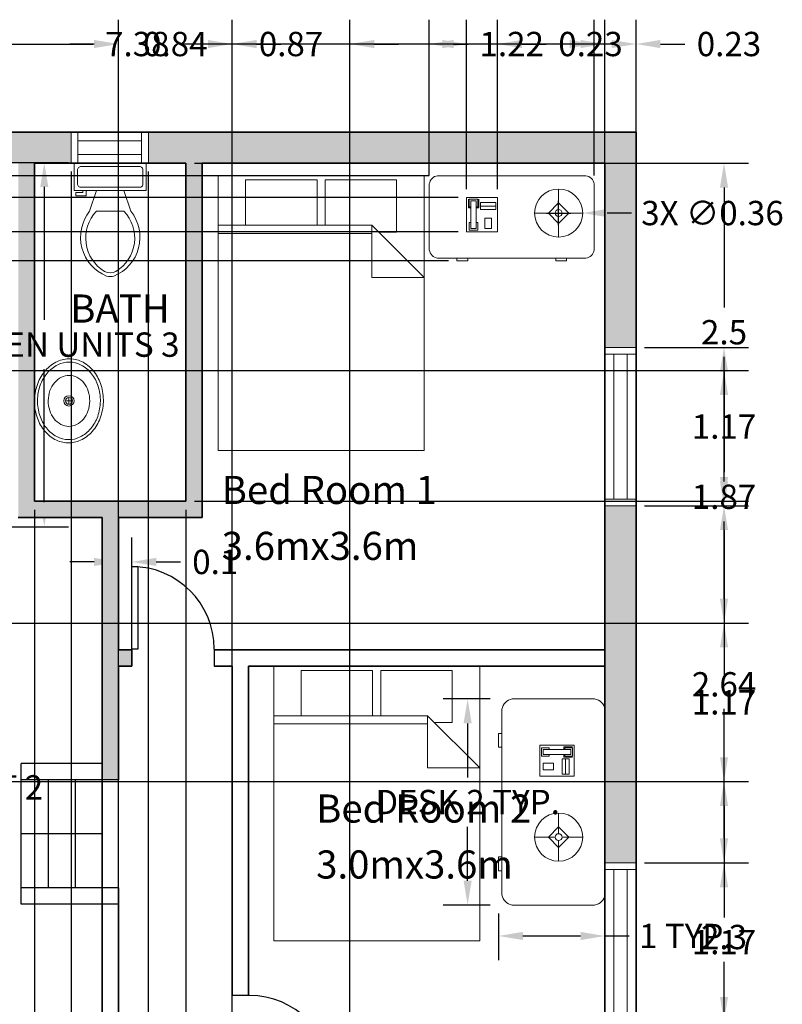
# Model space of a CAD drawing. Units: metres. Extents: x 35.2 to 46.4, y 446.1 to 460.8.
# Tile 6 of 6: x 40.4 to 46.1, y 453.5 to 460.8. Entities that reach past the tile are written whole.
import ezdxf

# ---------------------------------------------------------------- set-up
doc = ezdxf.new("R2010")
doc.units = ezdxf.units.M
for name, color, linetype, lineweight in [('A-ANNO-DIMS', 2, 'Continuous', 18), ('A-AREA-IDEN', 7, 'Continuous', 18), ('A-DOOR', 3, 'Continuous', 25), ('A-EQPM', 8, 'Continuous', 13), ('A-FLOR-STRS', 7, 'Continuous', 25), ('A-GLAZ', 4, 'Continuous', 18), ('A-WALL', 7, 'Continuous', 35), ('A-WALL-PATT', 252, 'Continuous', 13), ('FURNITURE', 53, 'Continuous', 18), ('SANITARY', 151, 'Continuous', 18)]:
    doc.layers.add(name, color=color, linetype=linetype, lineweight=lineweight)
doc.styles.get("Standard").update_dxf_attribs({"font": 'calibri.ttf'})
doc.dimstyles.get("Standard").update_dxf_attribs({"dimtxt": 0.18, "dimasz": 0.18, "dimexe": 0.18, "dimexo": 0.0625, "dimgap": 0.09, "dimtad": 0, "dimtih": 1, "dimtoh": 1, "dimdec": 4, "dimzin": 0, "dimdsep": 46, "dimtxsty": 'Standard', "dimcen": 0.09, "dimadec": 0, "dimazin": 0, "dimtfac": 1, "dimtdec": 4, "dimtofl": 0, "dimtmove": 0, "dimatfit": 3, "dimfxl": 1, "dimtolj": 1, "dimtzin": 0, "dimarcsym": 0})

# ---------------------------------------------------------------- blocks, each defined once
blk = doc.blocks.new('*U2')
for p, q in [((0, 0), (0, -5)), ((24, 0), (24, -5))]:
    blk.add_line(p, q)
blk.add_lwpolyline([(0, 0), (0, 24), (1.75, 24), (1.75, 0)], close=True)
blk.add_arc((0, 0), 24, 0, 90)
blk = doc.blocks.new('Bed - Queen')
for p, q in [((0, -80.00003), (0, 0)), ((0, 0), (59.99999, 0)), ((59.99999, 0), (59.99999, -80.00003)), ((7.99999, -1.2), (28.79998, -1.2)), ((7.99999, -14.4), (7.99999, -1.2)), ((28.79998, -1.2), (28.79998, -14.4)), ((31.19999, -1.2), (51.99999, -1.2)), ((31.19999, -14.4), (31.19999, -1.2)), ((51.99999, -1.2), (51.99999, -16.4)), ((0, -14.4), (44.8, -14.4)), ((44.8, -16.8), (0, -16.8)), ((59.99999, -29.6), (44.8, -14.4)), ((44.8, -14.4), (44.8, -29.6)), ((51.99999, -16.4), (46.79936, -16.4)), ((44.8, -29.6), (59.99999, -29.6)), ((59.99999, -80.00003), (0, -80.00003))]:
    blk.add_line(p, q)
blk = doc.blocks.new('Desk - 30 x 60 in.')
for p, q in [((-26.999995, 0), (26.999995, 0)), ((-29.999995, -27), (-29.999995, -3)), ((29.999995, -3), (29.999995, -27)), ((26.999995, -30), (-26.999995, -30)), ((-20.000005, -30), (-20.000005, -31)), ((-20.000005, -31), (-16.000005, -31)), ((-16.000005, -31), (-16.000005, -30)), ((15.999995, -31), (15.999995, -30)), ((19.999995, -31), (15.999995, -31)), ((19.999995, -30), (19.999995, -31))]:
    blk.add_line(p, q)
for centre, start, end in [((-26.499995, -3.5), 98.1301, 171.8699), ((26.499995, -3.5), 8.130102, 81.8699), ((-26.499995, -26.5), 188.1301, 261.8699), ((26.499995, -26.5), 278.1301, 351.8699)]:
    blk.add_arc(centre, 3.535534, start, end)
blk = doc.blocks.new('Lamp - Table')
for p, q in [((0, 7), (0, 1)), ((0, 3), (-3, 0)), ((3, 0), (0, 3)), ((-1, 0), (-7, 0)), ((-3, 0), (0, -3)), ((0, -3), (3, 0)), ((1, 0), (7, 0)), ((0, -1), (0, -7))]:
    blk.add_line(p, q)
for radius in [7, 1]:
    blk.add_circle((0, 0), radius)
blk = doc.blocks.new('Phone - Desk')
for p, q in [((-4.5, -5), (-4.5, 5)), ((-4.5, 5), (4.5, 5)), ((-4, 4.5), (-4, 2)), ((-3.75, 4.5), (-3.75, 2.25)), ((-1.25, 4.5), (-3.75, 4.5)), ((-3.25, 4), (-3.25, -4)), ((-3.25, 4), (-1.75, 4)), ((-1.75, -4), (-1.75, 4)), ((-1.25, 2.25), (-1.25, 4.5)), ((-1, 2), (-1, 4.5)), ((4, 3.5), (-0.5, 3.5)), ((-0.5, 3.5), (-0.5, 1.5)), ((4, 1.5), (4, 3.5)), ((4.5, 5), (4.5, -5)), ((-4, 2), (-3.25, 2)), ((-3.75, 2.25), (-3.25, 2.25)), ((-1.75, 2.25), (-1.25, 2.25)), ((-1.75, 2), (-1, 2)), ((-0.5, 2.5), (4, 2.5)), ((-0.5, 1.5), (4, 1.5)), ((-3.75, -2.25), (-3.25, -2.25)), ((-3.75, -4.5), (-3.75, -2.25)), ((-1.75, -2.25), (-1.25, -2.25)), ((-1.25, -2.25), (-1.25, -4.5)), ((2.75, -1), (0.75, -1)), ((0.75, -1), (0.75, -4)), ((2.75, -4), (2.75, -1)), ((4.5, -5), (-4.5, -5)), ((-1.25, -4.5), (-3.75, -4.5)), ((-3.25, -4), (-1.75, -4)), ((0.75, -4), (2.75, -4))]:
    blk.add_line(p, q)
blk = doc.blocks.new('Toilet - top')
for p, q in [((9.5, -6), (9.5, -2)), ((-10, -8.5), (-8, -8.5)), ((-10, -9.5), (-10, -8.5)), ((-8, -8.5), (-8, -8)), ((-7, -8), (-7, -9.5)), ((-4, -8), (-6, -14)), ((4, -8), (6, -14)), ((-7, -9.5), (-10, -9.5)), ((4, -14), (-4, -14))]:
    blk.add_line(p, q)
blk.add_lwpolyline([(10.5, -8), (10.5, 0), (-10.5, 0), (-10.5, -8)], close=True)
for points in [[(-9.5, -2), (-9.5, -6)], [(8.5, -1), (-8.5, -1)], [(-8.5, -7), (8.5, -7)]]:
    blk.add_lwpolyline(points)
for centre, radius, start, end in [((-8.62, -1.88), 0.884, 81.8699, 188.1301), ((8.62, -1.88), 0.884, 351.8699, 98.1301), ((-8.62, -6.12), 0.884, 171.8699, 278.1301), ((8.62, -6.12), 0.884, 261.8699, 8.1301), ((3.52, -21.58), 12.17, 141.4691, 247.9714), ((4.2, -21.82), 11.33, 136.3677, 238.9468), ((-3.52, -21.58), 12.17, 292.0284, 38.5307), ((-4.2, -21.82), 11.33, 301.053, 43.6321), ((0, -27.88), 4, 245.7318, 294.2682), ((0, -29), 4, 254.8605, 285.1395)]:
    blk.add_arc(centre, radius, start, end)
blk = doc.blocks.new('Sink - Oval top')
for p, q in [((-1, 0), (1, 0)), ((0, 1), (0, -1))]:
    blk.add_line(p, q)
for points in [[(-12.23, 0.39, 0.117634), (-11.46, -3.36, 0.104469), (-8.88, -6.8, 0.090016), (-5.08, -9.07, 0.08192), (-0.32, -10.02, 0.08192), (4.49, -9.38, 0.090016), (8.42, -7.36, 0.104469), (11.22, -4.09, 0.117634), (12.23, -0.39, 0.117634), (11.46, 3.36, 0.104469), (8.88, 6.8, 0.090016), (5.08, 9.07, 0.08192), (0.32, 10.02, 0.08192), (-4.49, 9.38, 0.090016), (-8.42, 7.36, 0.104469), (-11.22, 4.09, 0.117634)], [(-11.29, 0.16, 0.118622), (-10.52, -3.25, 0.104678), (-8.07, -6.36, 0.089562), (-4.54, -8.37, 0.081185), (-0.13, -9.15, 0.081185), (4.3, -8.49, 0.089562), (7.89, -6.58, 0.104678), (10.42, -3.55, 0.118622), (11.29, -0.16, 0.118622), (10.52, 3.25, 0.104678), (8.07, 6.36, 0.089562), (4.54, 8.37, 0.081185), (0.13, 9.15, 0.081185), (-4.3, 8.49, 0.089562), (-7.89, 6.58, 0.104678), (-10.42, 3.55, 0.118622)], [(-7.42, 0.08, 0.118283), (-6.91, -2.17, 0.104607), (-5.29, -4.21, 0.089718), (-2.97, -5.53, 0.081436), (-0.07, -6.04, 0.081436), (2.84, -5.59, 0.089718), (5.2, -4.33, 0.104607), (6.86, -2.32, 0.118283), (7.42, -0.08, 0.118283), (6.91, 2.17, 0.104607), (5.29, 4.21, 0.089718), (2.97, 5.53, 0.081436), (0.07, 6.04, 0.081436), (-2.84, 5.59, 0.089718), (-5.2, 4.33, 0.104607), (-6.86, 2.32, 0.118283)]]:
    blk.add_lwpolyline(points, format="xyb", close=True)
for radius in [1.5, 1]:
    blk.add_circle((0, 0), radius)
blk = doc.blocks.new('*U3')
for p, q in [((0, 0), (0, 5)), ((24, 0), (24, 5))]:
    blk.add_line(p, q)
blk.add_lwpolyline([(0, 0), (0, -24), (1.75, -24), (1.75, 0)], close=True)
blk.add_arc((0, 0), 24, 270, 0)
blk = doc.blocks.new('WIN-1172')
for p, q in [((0, 1.1716), (0.23, 1.1716)), ((0, 1.1716), (0, 0)), ((0.23, 1.1716), (0.23, 0)), ((0, 1.1216), (0.23, 1.1216)), ((0.065, 1.1216), (0.065, 0.05)), ((0.165, 1.1216), (0.165, 0.05)), ((0.23, 0.05), (0, 0.05)), ((0.23, 0), (0, 0))]:
    blk.add_line(p, q)
blk = doc.blocks.new('WIN-572')
for p, q in [((0, 0.5716), (0.23, 0.5716)), ((0, 0.5716), (0, 0)), ((0, 0.5216), (0.23, 0.5216)), ((0.065, 0.5216), (0.065, 0.05)), ((0.165, 0.5216), (0.165, 0.05)), ((0.23, 0.5716), (0.23, 0)), ((0.23, 0.05), (0, 0.05)), ((0.23, 0), (0, 0))]:
    blk.add_line(p, q)
blk = doc.blocks.new('*D133')
at = {"layer": 'A-ANNO-DIMS', "color": 0, "lineweight": -2, "transparency": 16777216}
for p, q in [((43.9067, 455.7324), (43.5606, 455.7324)), ((43.7406, 455.5524), (43.7406, 455.1526)), ((43.7406, 454.3884), (43.7406, 454.7882)), ((43.9067, 454.2084), (43.5606, 454.2084))]:
    blk.add_line(p, q, dxfattribs=at)
at = {"layer": 'A-ANNO-DIMS', "color": 0, "transparency": 16777216}
for points in [[(43.7106, 455.5524), (43.7706, 455.5524), (43.7406, 455.7324)], [(43.7106, 454.3884), (43.7706, 454.3884), (43.7406, 454.2084)]]:
    blk.add_solid(points, dxfattribs=at)
at = {"layer": 'Defpoints', "color": 0, "transparency": 16777216}
for p in [(43.9692, 455.7324), (43.7406, 454.2084), (43.9692, 454.2084)]:
    blk.add_point(p, dxfattribs=at)
at = {"layer": 'A-ANNO-DIMS', "color": 0, "transparency": 16777216, "insert": (43.7406, 454.9704), "char_height": 0.18, "attachment_point": 5}
blk.add_mtext('\\A1;DESK 2 TYP.', dxfattribs=at)
blk = doc.blocks.new('*D134')
at = {"layer": 'A-ANNO-DIMS', "color": 0, "lineweight": -2, "transparency": 16777216}
for p, q in [((43.9692, 454.1459), (43.9692, 453.7998)), ((44.7566, 454.1459), (44.7566, 453.7998)), ((44.1492, 453.9798), (44.5766, 453.9798)), ((44.7566, 453.9798), (44.9366, 453.9798))]:
    blk.add_line(p, q, dxfattribs=at)
at = {"layer": 'A-ANNO-DIMS', "color": 0, "transparency": 16777216}
for points in [[(44.1492, 454.0098), (44.1492, 453.9498), (43.9692, 453.9798)], [(44.5766, 454.0098), (44.5766, 453.9498), (44.7566, 453.9798)]]:
    blk.add_solid(points, dxfattribs=at)
at = {"layer": 'Defpoints', "color": 0, "transparency": 16777216}
for p in [(43.9692, 454.2084), (44.7566, 454.2084), (44.7566, 453.9798)]:
    blk.add_point(p, dxfattribs=at)
at = {"layer": 'A-ANNO-DIMS', "color": 0, "transparency": 16777216, "insert": (45.3552, 453.9798), "char_height": 0.18, "attachment_point": 5}
blk.add_mtext('\\A1;1 TYP.', dxfattribs=at)
blk = doc.blocks.new('*D139')
at = {"layer": 'A-ANNO-DIMS', "color": 0, "lineweight": -2, "transparency": 16777216}
for p, q in [((39.5553, 456.2345), (40.0195, 456.2345)), ((39.8395, 456.0545), (39.8395, 455.261)), ((39.8395, 454.1031), (39.8395, 454.8966)), ((39.5553, 453.9231), (40.0195, 453.9231))]:
    blk.add_line(p, q, dxfattribs=at)
at = {"layer": 'A-ANNO-DIMS', "color": 0, "transparency": 16777216}
for points in [[(39.8095, 456.0545), (39.8695, 456.0545), (39.8395, 456.2345)], [(39.8095, 454.1031), (39.8695, 454.1031), (39.8395, 453.9231)]]:
    blk.add_solid(points, dxfattribs=at)
at = {"layer": 'Defpoints', "color": 0, "transparency": 16777216}
for p in [(39.4928, 456.2345), (39.8395, 456.2345), (39.4928, 453.9231)]:
    blk.add_point(p, dxfattribs=at)
at = {"layer": 'A-ANNO-DIMS', "color": 0, "transparency": 16777216, "insert": (39.8395, 455.0788), "char_height": 0.18, "attachment_point": 5}
blk.add_mtext('\\A1;DINING SET 2', dxfattribs=at)
blk = doc.blocks.new('*D145')
at = {"layer": 'A-ANNO-DIMS', "color": 0, "lineweight": -2, "transparency": 16777216}
for p, q in [((40.2671, 459.6992), (40.7885, 459.6992)), ((40.6085, 459.5192), (40.6085, 458.5353)), ((40.6085, 457.1868), (40.6085, 458.1708)), ((40.2671, 457.0068), (40.7885, 457.0068))]:
    blk.add_line(p, q, dxfattribs=at)
at = {"layer": 'A-ANNO-DIMS', "color": 0, "transparency": 16777216}
for points in [[(40.5785, 459.5192), (40.6385, 459.5192), (40.6085, 459.6992)], [(40.5785, 457.1868), (40.6385, 457.1868), (40.6085, 457.0068)]]:
    blk.add_solid(points, dxfattribs=at)
at = {"layer": 'Defpoints', "color": 0, "transparency": 16777216}
for p in [(40.2046, 459.6992), (40.6085, 459.6992), (40.2046, 457.0068)]:
    blk.add_point(p, dxfattribs=at)
at = {"layer": 'A-ANNO-DIMS', "color": 0, "transparency": 16777216, "insert": (40.6085, 458.353), "char_height": 0.18, "attachment_point": 5}
blk.add_mtext('\\A1;KITCHEN UNITS 3', dxfattribs=at)
blk = doc.blocks.new('*D151')
at = {"layer": 'A-ANNO-DIMS', "color": 0, "lineweight": -2, "transparency": 16777216}
for p, q in [((37.6066, 459.9873), (37.6066, 460.756)), ((44.9866, 459.9873), (44.9866, 460.756)), ((37.7866, 460.576), (40.9679, 460.576)), ((44.8066, 460.576), (41.6253, 460.576))]:
    blk.add_line(p, q, dxfattribs=at)
at = {"layer": 'A-ANNO-DIMS', "color": 0, "transparency": 16777216}
for points in [[(37.7866, 460.606), (37.7866, 460.546), (37.6066, 460.576)], [(44.8066, 460.606), (44.8066, 460.546), (44.9866, 460.576)]]:
    blk.add_solid(points, dxfattribs=at)
at = {"layer": 'Defpoints', "color": 0, "transparency": 16777216}
for p in [(44.9866, 460.576), (37.6066, 459.9248), (44.9866, 459.9248)]:
    blk.add_point(p, dxfattribs=at)
at = {"layer": 'A-ANNO-DIMS', "color": 0, "transparency": 16777216, "insert": (41.2966, 460.576), "char_height": 0.18, "attachment_point": 5}
blk.add_mtext('\\A1;7.38', dxfattribs=at)
blk = doc.blocks.new('*D156')
at = {"layer": 'A-ANNO-DIMS', "color": 0, "lineweight": -2, "transparency": 16777216}
for p, q in [((37.8991, 455.122), (45.8178, 455.122)), ((45.6378, 454.942), (45.6378, 454.1543)), ((45.6378, 453.0022), (45.6378, 453.7898)), ((37.8991, 452.8222), (45.8178, 452.8222))]:
    blk.add_line(p, q, dxfattribs=at)
at = {"layer": 'A-ANNO-DIMS', "color": 0, "transparency": 16777216}
for points in [[(45.6078, 454.942), (45.6678, 454.942), (45.6378, 455.122)], [(45.6078, 453.0022), (45.6678, 453.0022), (45.6378, 452.8222)]]:
    blk.add_solid(points, dxfattribs=at)
at = {"layer": 'Defpoints', "color": 0, "transparency": 16777216}
for p in [(37.8366, 455.122), (45.6378, 455.122), (37.8366, 452.8222)]:
    blk.add_point(p, dxfattribs=at)
at = {"layer": 'A-ANNO-DIMS', "color": 0, "transparency": 16777216, "insert": (45.6378, 453.9721), "char_height": 0.18, "attachment_point": 5}
blk.add_mtext('\\A1;2.3', dxfattribs=at)
blk = doc.blocks.new('*D157')
at = {"layer": 'A-ANNO-DIMS', "color": 0, "lineweight": -2, "transparency": 16777216}
for p, q in [((37.8991, 456.2935), (45.8178, 456.2935)), ((45.6378, 456.1135), (45.6378, 455.8886)), ((45.6378, 455.302), (45.6378, 455.5269)), ((37.8991, 455.122), (45.8178, 455.122))]:
    blk.add_line(p, q, dxfattribs=at)
at = {"layer": 'A-ANNO-DIMS', "color": 0, "transparency": 16777216}
for points in [[(45.6078, 456.1135), (45.6678, 456.1135), (45.6378, 456.2935)], [(45.6078, 455.302), (45.6678, 455.302), (45.6378, 455.122)]]:
    blk.add_solid(points, dxfattribs=at)
at = {"layer": 'Defpoints', "color": 0, "transparency": 16777216}
for p in [(37.8366, 456.2935), (45.6378, 456.2935), (37.8366, 455.122)]:
    blk.add_point(p, dxfattribs=at)
at = {"layer": 'A-ANNO-DIMS', "color": 0, "transparency": 16777216, "insert": (45.6378, 455.7077), "char_height": 0.18, "attachment_point": 5}
blk.add_mtext('\\A1;1.17', dxfattribs=at)
blk = doc.blocks.new('*D158')
at = {"layer": 'A-ANNO-DIMS', "color": 0, "lineweight": -2, "transparency": 16777216}
for p, q in [((37.8991, 458.1617), (45.8178, 458.1617)), ((45.6378, 457.9817), (45.6378, 457.4098)), ((45.6378, 456.4735), (45.6378, 457.0454)), ((37.8991, 456.2935), (45.8178, 456.2935))]:
    blk.add_line(p, q, dxfattribs=at)
at = {"layer": 'A-ANNO-DIMS', "color": 0, "transparency": 16777216}
for points in [[(45.6078, 457.9817), (45.6678, 457.9817), (45.6378, 458.1617)], [(45.6078, 456.4735), (45.6678, 456.4735), (45.6378, 456.2935)]]:
    blk.add_solid(points, dxfattribs=at)
at = {"layer": 'Defpoints', "color": 0, "transparency": 16777216}
for p in [(37.8366, 458.1617), (45.6378, 458.1617), (37.8366, 456.2935)]:
    blk.add_point(p, dxfattribs=at)
at = {"layer": 'A-ANNO-DIMS', "color": 0, "transparency": 16777216, "insert": (45.6378, 457.2276), "char_height": 0.18, "attachment_point": 5}
blk.add_mtext('\\A1;1.87', dxfattribs=at)
blk = doc.blocks.new('*D164')
at = {"layer": 'A-ANNO-DIMS', "color": 0, "lineweight": -2, "transparency": 16777216}
for p, q in [((45.0491, 454.5208), (45.8178, 454.5208)), ((45.6378, 454.3408), (45.6378, 454.1159)), ((45.6378, 453.5293), (45.6378, 453.7542)), ((45.0491, 453.3493), (45.8178, 453.3493))]:
    blk.add_line(p, q, dxfattribs=at)
at = {"layer": 'A-ANNO-DIMS', "color": 0, "transparency": 16777216}
for points in [[(45.6078, 454.3408), (45.6678, 454.3408), (45.6378, 454.5208)], [(45.6078, 453.5293), (45.6678, 453.5293), (45.6378, 453.3493)]]:
    blk.add_solid(points, dxfattribs=at)
at = {"layer": 'Defpoints', "color": 0, "transparency": 16777216}
for p in [(44.9866, 454.5208), (45.6378, 454.5208), (44.9866, 453.3493)]:
    blk.add_point(p, dxfattribs=at)
at = {"layer": 'A-ANNO-DIMS', "color": 0, "transparency": 16777216, "insert": (45.6378, 453.9351), "char_height": 0.18, "attachment_point": 5}
blk.add_mtext('\\A1;1.17', dxfattribs=at)
blk = doc.blocks.new('*D165')
at = {"layer": 'A-ANNO-DIMS', "color": 0, "lineweight": -2, "transparency": 16777216}
for p, q in [((45.0491, 457.1611), (45.8178, 457.1611)), ((45.6378, 456.9811), (45.6378, 456.0232)), ((45.6378, 454.7008), (45.6378, 455.6588)), ((45.0491, 454.5208), (45.8178, 454.5208))]:
    blk.add_line(p, q, dxfattribs=at)
at = {"layer": 'A-ANNO-DIMS', "color": 0, "transparency": 16777216}
for points in [[(45.6078, 456.9811), (45.6678, 456.9811), (45.6378, 457.1611)], [(45.6078, 454.7008), (45.6678, 454.7008), (45.6378, 454.5208)]]:
    blk.add_solid(points, dxfattribs=at)
at = {"layer": 'Defpoints', "color": 0, "transparency": 16777216}
for p in [(44.9866, 457.1611), (45.6378, 457.1611), (44.9866, 454.5208)]:
    blk.add_point(p, dxfattribs=at)
at = {"layer": 'A-ANNO-DIMS', "color": 0, "transparency": 16777216, "insert": (45.6378, 455.841), "char_height": 0.18, "attachment_point": 5}
blk.add_mtext('\\A1;2.64', dxfattribs=at)
blk = doc.blocks.new('*D166')
at = {"layer": 'A-ANNO-DIMS', "color": 0, "lineweight": -2, "transparency": 16777216}
for p, q in [((45.0491, 458.3327), (45.8178, 458.3327)), ((45.6378, 458.1527), (45.6378, 457.9277)), ((45.6378, 457.3411), (45.6378, 457.5661)), ((45.0491, 457.1611), (45.8178, 457.1611))]:
    blk.add_line(p, q, dxfattribs=at)
at = {"layer": 'A-ANNO-DIMS', "color": 0, "transparency": 16777216}
for points in [[(45.6078, 458.1527), (45.6678, 458.1527), (45.6378, 458.3327)], [(45.6078, 457.3411), (45.6678, 457.3411), (45.6378, 457.1611)]]:
    blk.add_solid(points, dxfattribs=at)
at = {"layer": 'Defpoints', "color": 0, "transparency": 16777216}
for p in [(44.9866, 458.3327), (45.6378, 458.3327), (44.9866, 457.1611)]:
    blk.add_point(p, dxfattribs=at)
at = {"layer": 'A-ANNO-DIMS', "color": 0, "transparency": 16777216, "insert": (45.6378, 457.7469), "char_height": 0.18, "attachment_point": 5}
blk.add_mtext('\\A1;1.17', dxfattribs=at)
blk = doc.blocks.new('*D167')
at = {"layer": 'A-ANNO-DIMS', "color": 0, "lineweight": -2, "transparency": 16777216}
for p, q in [((37.8366, 459.6323), (37.8366, 446.0736)), ((40.8069, 459.6323), (40.8069, 446.0736)), ((38.0166, 446.2536), (38.9948, 446.2536)), ((40.6269, 446.2536), (39.6486, 446.2536))]:
    blk.add_line(p, q, dxfattribs=at)
at = {"layer": 'A-ANNO-DIMS', "color": 0, "transparency": 16777216}
for points in [[(38.0166, 446.2836), (38.0166, 446.2236), (37.8366, 446.2536)], [(40.6269, 446.2836), (40.6269, 446.2236), (40.8069, 446.2536)]]:
    blk.add_solid(points, dxfattribs=at)
at = {"layer": 'Defpoints', "color": 0, "transparency": 16777216}
for p in [(37.8366, 459.6948), (40.8069, 459.6948), (40.8069, 446.2536)]:
    blk.add_point(p, dxfattribs=at)
at = {"layer": 'A-ANNO-DIMS', "color": 0, "transparency": 16777216, "insert": (39.3217, 446.2536), "char_height": 0.18, "attachment_point": 5}
blk.add_mtext('\\A1;2.97', dxfattribs=at)
blk = doc.blocks.new('*D168')
at = {"layer": 'A-ANNO-DIMS', "color": 0, "lineweight": -2, "transparency": 16777216}
for p, q in [((40.8069, 459.6323), (40.8069, 446.0736)), ((41.3784, 459.6323), (41.3784, 446.0736)), ((40.9869, 446.2536), (41.1984, 446.2536)), ((41.3784, 446.2536), (41.5584, 446.2536))]:
    blk.add_line(p, q, dxfattribs=at)
at = {"layer": 'A-ANNO-DIMS', "color": 0, "transparency": 16777216}
for points in [[(40.9869, 446.2836), (40.9869, 446.2236), (40.8069, 446.2536)], [(41.1984, 446.2836), (41.1984, 446.2236), (41.3784, 446.2536)]]:
    blk.add_solid(points, dxfattribs=at)
at = {"layer": 'Defpoints', "color": 0, "transparency": 16777216}
for p in [(40.8069, 459.6948), (41.3784, 459.6948), (41.3784, 446.2536)]:
    blk.add_point(p, dxfattribs=at)
at = {"layer": 'A-ANNO-DIMS', "color": 0, "transparency": 16777216, "insert": (41.8883, 446.2536), "char_height": 0.18, "attachment_point": 5}
blk.add_mtext('\\A1;0.57', dxfattribs=at)
blk = doc.blocks.new('*D169')
at = {"layer": 'A-ANNO-DIMS', "color": 0, "lineweight": -2, "transparency": 16777216}
for p, q in [((40.536595, 457.132279), (40.536595, 446.073579)), ((41.656595, 457.132279), (41.656595, 446.073579)), ((40.356595, 446.253579), (40.176595, 446.253579)), ((41.836595, 446.253579), (42.016595, 446.253579))]:
    blk.add_line(p, q, dxfattribs=at)
at = {"layer": 'A-ANNO-DIMS', "color": 0, "transparency": 16777216}
for points in [[(40.356595, 446.283579), (40.356595, 446.223579), (40.536595, 446.253579)], [(41.836595, 446.283579), (41.836595, 446.223579), (41.656595, 446.253579)]]:
    blk.add_solid(points, dxfattribs=at)
at = {"layer": 'Defpoints', "color": 0, "transparency": 16777216}
for p in [(40.536595, 457.194779), (41.656595, 457.194779), (41.656595, 446.253579)]:
    blk.add_point(p, dxfattribs=at)
at = {"layer": 'A-ANNO-DIMS', "color": 0, "transparency": 16777216, "insert": (41.096595, 446.253579), "char_height": 0.18, "attachment_point": 5}
blk.add_mtext('\\A1;1.12', dxfattribs=at)
blk = doc.blocks.new('*D170')
at = {"layer": 'A-ANNO-DIMS', "color": 0, "lineweight": -2, "transparency": 16777216}
for p, q in [((41.7191, 459.6948), (45.8178, 459.6948)), ((45.6378, 459.5148), (45.6378, 458.627)), ((45.6378, 457.3748), (45.6378, 458.2626)), ((41.7191, 457.1948), (45.8178, 457.1948))]:
    blk.add_line(p, q, dxfattribs=at)
at = {"layer": 'A-ANNO-DIMS', "color": 0, "transparency": 16777216}
for points in [[(45.6078, 459.5148), (45.6678, 459.5148), (45.6378, 459.6948)], [(45.6078, 457.3748), (45.6678, 457.3748), (45.6378, 457.1948)]]:
    blk.add_solid(points, dxfattribs=at)
at = {"layer": 'Defpoints', "color": 0, "transparency": 16777216}
for p in [(41.6566, 459.6948), (41.6566, 457.1948), (45.6378, 457.1948)]:
    blk.add_point(p, dxfattribs=at)
at = {"layer": 'A-ANNO-DIMS', "color": 0, "transparency": 16777216, "insert": (45.6378, 458.4448), "char_height": 0.18, "attachment_point": 5}
blk.add_mtext('\\A1;2.5', dxfattribs=at)
blk = doc.blocks.new('*D175')
at = {"layer": 'A-ANNO-DIMS', "color": 0, "lineweight": -2, "transparency": 16777216}
for p, q in [((44.7566, 451.1428), (44.7566, 460.756)), ((44.9866, 451.1428), (44.9866, 460.756)), ((44.5766, 460.576), (44.3966, 460.576)), ((45.1666, 460.576), (45.3466, 460.576))]:
    blk.add_line(p, q, dxfattribs=at)
at = {"layer": 'A-ANNO-DIMS', "color": 0, "transparency": 16777216}
for points in [[(44.5766, 460.606), (44.5766, 460.546), (44.7566, 460.576)], [(45.1666, 460.606), (45.1666, 460.546), (44.9866, 460.576)]]:
    blk.add_solid(points, dxfattribs=at)
at = {"layer": 'Defpoints', "color": 0, "transparency": 16777216}
for p in [(44.9866, 460.576), (44.7566, 451.0803), (44.9866, 451.0803)]:
    blk.add_point(p, dxfattribs=at)
at = {"layer": 'A-ANNO-DIMS', "color": 0, "transparency": 16777216, "insert": (45.6744, 460.576), "char_height": 0.18, "attachment_point": 5}
blk.add_mtext('\\A1;0.23', dxfattribs=at)
blk = doc.blocks.new('*D176')
at = {"layer": 'A-ANNO-DIMS', "color": 0, "lineweight": -2, "transparency": 16777216}
for p, q in [((43.7336, 459.5036), (43.7336, 460.756)), ((43.9622, 459.5036), (43.9622, 460.756)), ((43.5536, 460.576), (43.3736, 460.576)), ((44.1422, 460.576), (44.3222, 460.576))]:
    blk.add_line(p, q, dxfattribs=at)
at = {"layer": 'A-ANNO-DIMS', "color": 0, "transparency": 16777216}
for points in [[(43.5536, 460.606), (43.5536, 460.546), (43.7336, 460.576)], [(44.1422, 460.606), (44.1422, 460.546), (43.9622, 460.576)]]:
    blk.add_solid(points, dxfattribs=at)
at = {"layer": 'Defpoints', "color": 0, "transparency": 16777216}
for p in [(43.9622, 460.576), (43.7336, 459.4411), (43.9622, 459.4411)]:
    blk.add_point(p, dxfattribs=at)
at = {"layer": 'A-ANNO-DIMS', "color": 0, "transparency": 16777216, "insert": (44.65, 460.576), "char_height": 0.18, "attachment_point": 5}
blk.add_mtext('\\A1;0.23', dxfattribs=at)
blk = doc.blocks.new('*D177')
at = {"layer": 'A-ANNO-DIMS', "color": 0, "lineweight": -2, "transparency": 16777216}
for p, q in [((36.9554, 459.6211), (36.9554, 459.8011)), ((36.9554, 459.8011), (37.1354, 459.8011)), ((43.6711, 459.4411), (36.7754, 459.4411)), ((43.6711, 459.1871), (36.7754, 459.1871)), ((36.9554, 459.0071), (36.9554, 458.8271))]:
    blk.add_line(p, q, dxfattribs=at)
at = {"layer": 'A-ANNO-DIMS', "color": 0, "transparency": 16777216}
for points in [[(36.9254, 459.6211), (36.9854, 459.6211), (36.9554, 459.4411)], [(36.9254, 459.0071), (36.9854, 459.0071), (36.9554, 459.1871)]]:
    blk.add_solid(points, dxfattribs=at)
at = {"layer": 'Defpoints', "color": 0, "transparency": 16777216}
for p in [(36.9554, 459.4411), (43.7336, 459.4411), (43.7336, 459.1871)]:
    blk.add_point(p, dxfattribs=at)
at = {"layer": 'A-ANNO-DIMS', "color": 0, "transparency": 16777216, "insert": (37.5396, 459.8011), "char_height": 0.18, "attachment_point": 5}
blk.add_mtext('\\A1;0.254', dxfattribs=at)
blk = doc.blocks.new('*D178')
at = {"layer": 'A-ANNO-DIMS', "color": 0, "lineweight": -2, "transparency": 16777216}
for p, q in [((43.4574, 459.6039), (43.4574, 460.756)), ((44.6766, 459.6039), (44.6766, 460.756)), ((43.6374, 460.576), (43.7456, 460.576)), ((44.4966, 460.576), (44.3884, 460.576))]:
    blk.add_line(p, q, dxfattribs=at)
at = {"layer": 'A-ANNO-DIMS', "color": 0, "transparency": 16777216}
for points in [[(43.6374, 460.606), (43.6374, 460.546), (43.4574, 460.576)], [(44.4966, 460.606), (44.4966, 460.546), (44.6766, 460.576)]]:
    blk.add_solid(points, dxfattribs=at)
at = {"layer": 'Defpoints', "color": 0, "transparency": 16777216}
for p in [(44.6766, 460.576), (43.4574, 459.5414), (44.6766, 459.5414)]:
    blk.add_point(p, dxfattribs=at)
at = {"layer": 'A-ANNO-DIMS', "color": 0, "transparency": 16777216, "insert": (44.067, 460.576), "char_height": 0.18, "attachment_point": 5}
blk.add_mtext('\\A1;1.22', dxfattribs=at)
blk = doc.blocks.new('*D179')
at = {"layer": 'A-ANNO-DIMS', "color": 0, "lineweight": -2, "transparency": 16777216}
for p, q in [((43.4559, 459.6024), (36.7754, 459.6024)), ((36.9554, 459.4224), (36.9554, 459.1525)), ((43.5981, 458.9725), (36.7754, 458.9725)), ((36.9554, 458.9725), (36.9554, 458.7925)), ((36.9554, 458.7925), (36.7754, 458.7925))]:
    blk.add_line(p, q, dxfattribs=at)
at = {"layer": 'A-ANNO-DIMS', "color": 0, "transparency": 16777216}
for points in [[(36.9254, 459.4224), (36.9854, 459.4224), (36.9554, 459.6024)], [(36.9254, 459.1525), (36.9854, 459.1525), (36.9554, 458.9725)]]:
    blk.add_solid(points, dxfattribs=at)
at = {"layer": 'Defpoints', "color": 0, "transparency": 16777216}
for p in [(43.5184, 459.6024), (36.9554, 458.9725), (43.6606, 458.9725)]:
    blk.add_point(p, dxfattribs=at)
at = {"layer": 'A-ANNO-DIMS', "color": 0, "transparency": 16777216, "insert": (36.4476, 458.7925), "char_height": 0.18, "attachment_point": 5}
blk.add_mtext('\\A1;0.63', dxfattribs=at)
blk = doc.blocks.new('*D182')
at = {"layer": 'A-ANNO-DIMS', "color": 0, "lineweight": -2, "transparency": 16777216}
for p, q in [((41.9991, 452.3173), (41.9991, 460.756)), ((42.8695, 452.3173), (42.8695, 460.756)), ((41.8191, 460.576), (41.6391, 460.576)), ((43.0495, 460.576), (43.2295, 460.576))]:
    blk.add_line(p, q, dxfattribs=at)
at = {"layer": 'A-ANNO-DIMS', "color": 0, "transparency": 16777216}
for points in [[(41.8191, 460.606), (41.8191, 460.546), (41.9991, 460.576)], [(43.0495, 460.606), (43.0495, 460.546), (42.8695, 460.576)]]:
    blk.add_solid(points, dxfattribs=at)
at = {"layer": 'Defpoints', "color": 0, "transparency": 16777216}
for p in [(42.8695, 460.576), (41.9991, 452.2548), (42.8695, 452.2548)]:
    blk.add_point(p, dxfattribs=at)
at = {"layer": 'A-ANNO-DIMS', "color": 0, "transparency": 16777216, "insert": (42.4343, 460.576), "char_height": 0.18, "attachment_point": 5}
blk.add_mtext('\\A1;0.87', dxfattribs=at)
blk = doc.blocks.new('*D183')
at = {"layer": 'A-ANNO-DIMS', "color": 0, "lineweight": -2, "transparency": 16777216}
for p, q in [((41.1566, 450.3173), (41.1566, 460.756)), ((41.9991, 450.3173), (41.9991, 460.756)), ((40.9766, 460.576), (40.7966, 460.576)), ((42.1791, 460.576), (42.3591, 460.576))]:
    blk.add_line(p, q, dxfattribs=at)
at = {"layer": 'A-ANNO-DIMS', "color": 0, "transparency": 16777216}
for points in [[(40.9766, 460.606), (40.9766, 460.546), (41.1566, 460.576)], [(42.1791, 460.606), (42.1791, 460.546), (41.9991, 460.576)]]:
    blk.add_solid(points, dxfattribs=at)
at = {"layer": 'Defpoints', "color": 0, "transparency": 16777216}
for p in [(41.9991, 460.576), (41.1566, 450.2548), (41.9991, 450.2548)]:
    blk.add_point(p, dxfattribs=at)
at = {"layer": 'A-ANNO-DIMS', "color": 0, "transparency": 16777216, "insert": (41.5779, 460.576), "char_height": 0.18, "attachment_point": 5}
blk.add_mtext('\\A1;0.84', dxfattribs=at)
blk = doc.blocks.new('*D184')
at = {"layer": 'A-ANNO-DIMS', "color": 0, "lineweight": -2, "transparency": 16777216}
for p, q in [((41.1566, 456.1573), (41.1566, 456.926)), ((41.2566, 456.1573), (41.2566, 456.926)), ((40.9766, 456.746), (40.7966, 456.746)), ((41.4366, 456.746), (41.6166, 456.746))]:
    blk.add_line(p, q, dxfattribs=at)
at = {"layer": 'A-ANNO-DIMS', "color": 0, "transparency": 16777216}
for points in [[(40.9766, 456.776), (40.9766, 456.716), (41.1566, 456.746)], [(41.4366, 456.776), (41.4366, 456.716), (41.2566, 456.746)]]:
    blk.add_solid(points, dxfattribs=at)
at = {"layer": 'Defpoints', "color": 0, "transparency": 16777216}
for p in [(41.2566, 456.746), (41.1566, 456.0948), (41.2566, 456.0948)]:
    blk.add_point(p, dxfattribs=at)
at = {"layer": 'A-ANNO-DIMS', "color": 0, "transparency": 16777216, "insert": (41.8734, 456.746), "char_height": 0.18, "attachment_point": 5}
blk.add_mtext('\\A1;0.1', dxfattribs=at)
blk = doc.blocks.new('*D192')
at = {"layer": 'A-ANNO-DIMS', "color": 0, "lineweight": -2, "transparency": 16777216}
for p, q in [((44.4142, 459.236), (44.4142, 459.416)), ((44.3242, 459.326), (44.5042, 459.326)), ((44.952, 459.326), (44.772, 459.326))]:
    blk.add_line(p, q, dxfattribs=at)
at = {"layer": 'A-ANNO-DIMS', "color": 0, "transparency": 16777216}
blk.add_solid([(44.772, 459.356), (44.772, 459.296), (44.592, 459.326)], dxfattribs=at)
at = {"layer": 'Defpoints', "color": 0, "transparency": 16777216}
for p in [(44.2364, 459.326), (44.592, 459.326)]:
    blk.add_point(p, dxfattribs=at)
at = {"layer": 'A-ANNO-DIMS', "color": 0, "transparency": 16777216, "insert": (45.5522, 459.326), "char_height": 0.18, "attachment_point": 5}
blk.add_mtext('\\A1;3X ∅0.36', dxfattribs=at)

msp = doc.modelspace()

# ---------------------------------------------------------------- hatches: boundary and pattern name
at = {"layer": 'A-WALL-PATT'}
h = msp.add_hatch(color=256, dxfattribs=at)
h.dxf.hatch_style = 1
h.paths.add_polyline_path([(37.8366, 451.6506), (37.6066, 451.6506), (37.6066, 449.5548), (40.327, 449.5548), (40.327, 449.6748), (37.8366, 449.6748)])
h.paths.add_polyline_path([(37.8366, 455.122), (37.6066, 455.122), (37.6066, 452.8222), (37.8366, 452.8222)])
h.paths.add_polyline_path([(37.8366, 457.0257), (37.8366, 457.0747), (37.8341, 457.0771), (37.8366, 457.0796), (37.8366, 457.1285), (37.8341, 457.131), (37.8366, 457.1335), (37.8366, 457.1824), (37.8341, 457.1849), (37.8366, 457.1874), (37.8366, 457.2363), (37.8341, 457.2388), (37.8366, 457.2412), (37.8366, 457.2902), (37.8341, 457.2927), (37.8366, 457.2951), (37.8366, 457.3441), (37.8341, 457.3465), (37.8366, 457.349), (37.8366, 457.398), (37.8341, 457.4004), (37.8366, 457.4029), (37.8366, 457.4518), (37.8341, 457.4543), (37.8366, 457.4568), (37.8366, 457.5057), (37.8341, 457.5082), (37.8366, 457.5107), (37.8366, 457.5596), (37.8341, 457.5621), (37.8366, 457.5645), (37.8366, 457.6135), (37.8341, 457.6159), (37.8366, 457.6184), (37.8366, 457.6674), (37.8341, 457.6698), (37.8366, 457.6723), (37.8366, 457.7212), (37.8341, 457.7237), (37.8366, 457.7262), (37.8366, 457.7751), (37.8341, 457.7776), (37.8366, 457.7801), (37.8366, 457.829), (37.8341, 457.8315), (37.8366, 457.8339), (37.8366, 457.8829), (37.8341, 457.8854), (37.8366, 457.8878), (37.8366, 457.9368), (37.8341, 457.9392), (37.8366, 457.9417), (37.8366, 457.9906), (37.8341, 457.9931), (37.8366, 457.9956), (37.8366, 458.0445), (37.8341, 458.047), (37.8366, 458.0495), (37.8366, 458.0984), (37.8341, 458.1009), (37.8366, 458.1033), (37.8366, 458.1523), (37.8272, 458.1617), (37.6066, 458.1617), (37.6066, 456.2935), (37.8366, 456.2935), (37.8366, 457.0208), (37.8341, 457.0232)], flags=17)
h.paths.add_polyline_path([(40.8069, 459.9248), (37.6066, 459.9248), (37.6066, 459.3333), (37.8273, 459.3333), (37.8366, 459.3426), (37.8366, 459.3916), (37.8341, 459.394), (37.8366, 459.3965), (37.8366, 459.4455), (37.8341, 459.4479), (37.8366, 459.4504), (37.8366, 459.4993), (37.8341, 459.5018), (37.8366, 459.5043), (37.8366, 459.5532), (37.8341, 459.5557), (37.8366, 459.5582), (37.8366, 459.6071), (37.8341, 459.6096), (37.8366, 459.612), (37.8366, 459.661), (37.8341, 459.6634), (37.8366, 459.6659), (37.8366, 459.6948), (40.4166, 459.6948), (40.4166, 457.0748), (41.0366, 457.0748), (41.0366, 455.1347), (41.1566, 455.1347), (41.1566, 455.9748), (41.2566, 455.9748), (41.2566, 456.0948), (41.1566, 456.0948), (41.1566, 457.0748), (41.7766, 457.0748), (41.7766, 459.6948), (44.7566, 459.6948), (44.7566, 458.3327), (44.9866, 458.3327), (44.9866, 459.9248), (41.3784, 459.9248), (41.3784, 459.6948), (41.6566, 459.6948), (41.6566, 457.1948), (40.5366, 457.1948), (40.5366, 459.6948), (40.8069, 459.6948)])
h.paths.add_polyline_path([(42.1191, 452.2548), (41.9991, 452.2548), (41.9991, 451.3542), (42.1191, 451.3542)])
h = msp.add_hatch(color=256, dxfattribs=at)
h.dxf.hatch_style = 1
h.paths.add_polyline_path([(44.9866, 457.1611), (44.7566, 457.1611), (44.7566, 454.5208), (44.9866, 454.5208)])
h.paths.add_polyline_path([(44.9866, 453.3493), (44.7566, 453.3493), (44.7566, 452.3748), (42.8766, 452.3748), (42.8766, 452.8748), (42.1191, 452.8748), (42.1191, 452.9307), (41.9991, 452.9307), (41.9991, 452.2548), (42.1191, 452.2548), (42.1191, 452.7548), (42.7566, 452.7548), (42.7566, 452.2548), (44.7566, 452.2548), (44.7566, 451.6519), (44.9866, 451.6519)])
h.paths.add_polyline_path([(44.9866, 451.0803), (44.7566, 451.0803), (44.7566, 450.2548), (43.6593, 450.2548), (43.0598, 450.2548, -0.016107), (43.0354, 450.2548), (42.1191, 450.2548), (42.1191, 450.7446), (41.9991, 450.7446), (41.9991, 450.2548), (41.8662, 450.2548), (41.8662, 450.1348), (44.7566, 450.1348), (44.7566, 448.5414), (44.9866, 448.5414)])
h.paths.add_polyline_path([(44.9866, 447.3698), (44.7566, 447.3698), (44.7566, 447.1348), (41.1566, 447.1348), (41.1566, 450.1348), (41.2566, 450.1348), (41.2566, 450.2548), (41.0366, 450.2548), (41.0366, 446.9048), (44.9866, 446.9048)])

# ---------------------------------------------------------------- linework, layer by layer
at = {"layer": 'A-FLOR-STRS'}
for p, q in [((40.4366, 454.2147), (40.4366, 455.2547)), ((41.0366, 455.2547), (40.4366, 455.2547)), ((41.1566, 455.1347), (40.4366, 455.1347)), ((40.6366, 455.1347), (40.6366, 454.3347)), ((40.8366, 455.1347), (40.8366, 454.3347)), ((41.0366, 454.7347), (40.4366, 454.7347)), ((41.1566, 454.3347), (40.4366, 454.3347)), ((41.1566, 454.2147), (40.4366, 454.2147))]:
    msp.add_line(p, q, dxfattribs=at)
at = {"layer": 'A-WALL'}
for p, q in [((37.6066, 459.9248), (44.9866, 459.9248)), ((44.9866, 459.9248), (44.9866, 446.9048)), ((40.5366, 459.6948), (40.5366, 457.1948)), ((40.5366, 459.6948), (41.6566, 459.6948)), ((41.6566, 459.6948), (41.6566, 457.1948)), ((41.7766, 459.6948), (41.7766, 457.0748)), ((41.7766, 459.6948), (44.7566, 459.6948)), ((44.7566, 459.6948), (44.7566, 452.3748)), ((40.5366, 457.1948), (41.6566, 457.1948)), ((40.4166, 457.0748), (41.0366, 457.0748)), ((41.0366, 454.2147), (41.0366, 457.0748)), ((41.1566, 457.0748), (41.1566, 456.0948)), ((41.1566, 457.0748), (41.7766, 457.0748)), ((41.1566, 456.0948), (41.2566, 456.0948)), ((41.2566, 456.0948), (41.2566, 455.9748)), ((41.8662, 456.0948), (44.7566, 456.0948)), ((41.1566, 455.9748), (41.2566, 455.9748)), ((41.1566, 455.9748), (41.1566, 455.1347)), ((41.8662, 455.9748), (41.9991, 455.9748)), ((41.9991, 455.9748), (41.9991, 453.5403)), ((42.1191, 455.9748), (42.1191, 453.5403)), ((42.1191, 455.9748), (44.7566, 455.9748))]:
    msp.add_line(p, q, dxfattribs=at)
at = {"layer": 'A-WALL', "transparency": 33554534}
for p, q in [((41.1566, 454.3347), (41.1566, 450.2548)), ((41.0366, 450.2548), (41.0366, 454.2147))]:
    msp.add_line(p, q, dxfattribs=at)

# ---------------------------------------------------------------- block references
at = {"layer": 'A-DOOR', "xscale": 0.0254, "yscale": 0.0254, "zscale": 0.0254}
msp.add_blockref('*U2', (41.2566, 456.1018), dxfattribs=at)
at = {"layer": 'A-DOOR', "xscale": 0.0254, "yscale": 0.0254, "zscale": 0.0254, "rotation": 90}
msp.add_blockref('*U3', (42.1261, 452.9307), dxfattribs=at)
at = {"layer": 'A-EQPM', "transparency": 33554521, "xscale": 0.0254, "yscale": 0.0254, "zscale": 0.0254}
for name, p in [('Lamp - Table', (44.4142, 459.326)), ('Phone - Desk', (43.8479, 459.3141))]:
    msp.add_blockref(name, p, dxfattribs=at)
at = {"layer": 'A-EQPM', "transparency": 33554521, "xscale": 0.0254, "yscale": 0.0254, "zscale": 0.0254, "rotation": 270}
for name, p in [('Phone - Desk', (44.4022, 455.2772)), ('Lamp - Table', (44.4142, 454.711))]:
    msp.add_blockref(name, p, dxfattribs=at)
at = {"layer": 'A-GLAZ', "rotation": 89.99999999998899}
msp.add_blockref('WIN-572', (41.3785, 459.6948), dxfattribs=at)
at = {"layer": 'A-GLAZ'}
for p in [(44.7566, 457.1611), (44.7566, 453.3493)]:
    msp.add_blockref('WIN-1172', p, dxfattribs=at)
at = {"layer": 'FURNITURE', "transparency": 33554457, "xscale": 0.0254, "yscale": 0.0254, "zscale": 0.0254}
msp.add_blockref('Bed - Queen', (41.8949, 459.6019), dxfattribs=at)
at = {"layer": 'FURNITURE', "transparency": 33554521}
for name, p, xscale, yscale, zscale in [('Desk - 30 x 60 in.', (44.067, 459.6024), 0.02032, 0.02032, 0.02032), ('Bed - Queen', (42.3065, 455.9748), 0.0254, 0.0254, 0.0254)]:
    msp.add_blockref(name, p, dxfattribs=dict(at, xscale=xscale, yscale=yscale, zscale=zscale))
at = {"layer": 'FURNITURE', "transparency": 33554521, "xscale": 0.0254, "yscale": 0.0254, "zscale": 0.0254, "rotation": 270}
msp.add_blockref('Desk - 30 x 60 in.', (44.7566, 454.9704), dxfattribs=at)
at = {"layer": 'SANITARY', "transparency": 33554521, "xscale": 0.0254, "yscale": 0.0254, "zscale": 0.0254}
msp.add_blockref('Toilet - top', (41.0966, 459.6948), dxfattribs=at)
at = {"layer": 'SANITARY', "transparency": 33554521, "xscale": 0.0254, "yscale": 0.0254, "zscale": 0.0254, "rotation": 90}
msp.add_blockref('Sink - Oval top', (40.7912, 457.9372), dxfattribs=at)

# ---------------------------------------------------------------- texts
at = {"layer": 'A-AREA-IDEN'}
for s, p in [('BATH', (40.8007, 458.5157)), ('Bed Room 1', (41.9213, 457.1743)), ('3.6mx3.6m', (41.9213, 456.7606)), ('Bed Room 2', (42.6201, 454.8182)), ('3.0mx3.6m', (42.6201, 454.4045))]:
    msp.add_text(s, height=0.20807, dxfattribs=at).set_placement(p)

# ---------------------------------------------------------------- dimensions: what is measured, and where the dimension line sits
at = {"layer": 'A-ANNO-DIMS'}
for base, p1, p2, override, picture, middle in [((44.9866, 460.576), (37.6066, 459.9248), (44.9866, 459.9248), {"dimdec": 2, "dimlfac": 1, "dimrnd": 0, "dimzin": 0, "dimdsep": 46, "dimlunit": 2}, '*D151', (41.2966, 460.576)), ((41.9991, 460.576), (41.1566, 450.2548), (41.9991, 450.2548), {"dimdec": 2, "dimlfac": 1, "dimrnd": 0, "dimzin": 0, "dimdsep": 46, "dimlunit": 2}, '*D183', (41.5779, 460.576)), ((42.8695, 460.576), (41.9991, 452.2548), (42.8695, 452.2548), {"dimdec": 2, "dimlfac": 1, "dimrnd": 0, "dimzin": 0, "dimdsep": 46, "dimlunit": 2}, '*D182', (42.4343, 460.576)), ((43.9622, 460.576), (43.7336, 459.4411), (43.9622, 459.4411), {"dimdec": 2, "dimlfac": 1, "dimrnd": 0, "dimzin": 0, "dimdsep": 46, "dimlunit": 2}, '*D176', (44.65, 460.576)), ((44.6766, 460.576), (43.4574, 459.5414), (44.6766, 459.5414), {"dimdec": 2, "dimlfac": 1, "dimrnd": 0, "dimzin": 0, "dimdsep": 46, "dimlunit": 2}, '*D178', (44.067, 460.576)), ((44.9866, 460.576), (44.7566, 451.0803), (44.9866, 451.0803), {"dimdec": 2, "dimlfac": 1, "dimrnd": 0, "dimzin": 0, "dimdsep": 46, "dimlunit": 2}, '*D175', (45.6744, 460.576)), ((40.8069, 446.2536), (37.8366, 459.6948), (40.8069, 459.6948), {"dimdec": 2, "dimlfac": 1, "dimrnd": 0, "dimzin": 0, "dimdsep": 46, "dimlunit": 2}, '*D167', (39.3217, 446.2536)), ((41.3784, 446.2536), (40.8069, 459.6948), (41.3784, 459.6948), {"dimdec": 2, "dimlfac": 1, "dimrnd": 0, "dimzin": 0, "dimdsep": 46, "dimlunit": 2}, '*D168', (41.8883, 446.2536)), ((41.6566, 446.2536), (40.5366, 457.1948), (41.6566, 457.1948), {"dimdec": 2, "dimlfac": 1, "dimrnd": 0, "dimzin": 0, "dimdsep": 46, "dimlunit": 2}, '*D169', (41.0966, 446.2536)), ((41.2566, 456.746), (41.1566, 456.0948), (41.2566, 456.0948), {"dimdec": 1, "dimlfac": 1, "dimrnd": 0, "dimzin": 0, "dimdsep": 46, "dimlunit": 2}, '*D184', (41.8734, 456.746))]:
    dim = msp.add_linear_dim(base=base, p1=p1, p2=p2, dimstyle='Standard', override=override, dxfattribs=at)
    dim.commit()
    dim.dimension.update_dxf_attribs({"geometry": picture, "text_midpoint": middle})
for base, p1, p2, override, picture, middle in [((36.9554, 459.4411), (43.7336, 459.1871), (43.7336, 459.4411), {"dimdec": 3, "dimlfac": 1, "dimrnd": 0, "dimzin": 0, "dimdsep": 46, "dimlunit": 2}, '*D177', (37.5396, 459.8011)), ((45.6378, 457.1948), (41.6566, 459.6948), (41.6566, 457.1948), {"dimdec": 1, "dimlfac": 1, "dimrnd": 0, "dimzin": 0, "dimdsep": 46, "dimlunit": 2}, '*D170', (45.6378, 458.4448)), ((36.9554, 458.9725), (43.5184, 459.6024), (43.6606, 458.9725), {"dimdec": 2, "dimlfac": 1, "dimrnd": 0, "dimzin": 0, "dimdsep": 46, "dimlunit": 2}, '*D179', (36.4476, 458.7925)), ((45.6378, 458.3327), (44.9866, 457.1611), (44.9866, 458.3327), {"dimdec": 2, "dimlfac": 1, "dimrnd": 0, "dimzin": 0, "dimdsep": 46, "dimlunit": 2}, '*D166', (45.6378, 457.7469)), ((45.6378, 458.1617), (37.8366, 456.2935), (37.8366, 458.1617), {"dimdec": 2, "dimlfac": 1, "dimrnd": 0, "dimzin": 0, "dimdsep": 46, "dimlunit": 2}, '*D158', (45.6378, 457.2276)), ((45.6378, 457.1611), (44.9866, 454.5208), (44.9866, 457.1611), {"dimdec": 2, "dimlfac": 1, "dimrnd": 0, "dimzin": 0, "dimdsep": 46, "dimlunit": 2}, '*D165', (45.6378, 455.841)), ((45.6378, 456.2935), (37.8366, 455.122), (37.8366, 456.2935), {"dimdec": 2, "dimlfac": 1, "dimrnd": 0, "dimzin": 0, "dimdsep": 46, "dimlunit": 2}, '*D157', (45.6378, 455.7077)), ((45.6378, 455.122), (37.8366, 452.8222), (37.8366, 455.122), {"dimdec": 1, "dimlfac": 1, "dimrnd": 0, "dimzin": 0, "dimdsep": 46, "dimlunit": 2}, '*D156', (45.6378, 453.9721)), ((45.6378, 454.5208), (44.9866, 453.3493), (44.9866, 454.5208), {"dimdec": 2, "dimlfac": 1, "dimrnd": 0, "dimzin": 0, "dimdsep": 46, "dimlunit": 2}, '*D164', (45.6378, 453.9351))]:
    dim = msp.add_linear_dim(base=base, p1=p1, p2=p2, angle=90, dimstyle='Standard', override=override, dxfattribs=at)
    dim.commit()
    dim.dimension.update_dxf_attribs({"geometry": picture, "text_midpoint": middle})
for base, p1, p2, angle, text, picture, middle in [((40.6085, 459.6992), (40.2046, 457.0068), (40.2046, 459.6992), 90, 'KITCHEN UNITS <>', '*D145', (40.6085, 458.353)), ((39.8395, 456.2345), (39.4928, 453.9231), (39.4928, 456.2345), 90, 'DINING SET <>', '*D139', (39.8395, 455.0788)), ((43.7406, 454.2084), (43.9692, 455.7324), (43.9692, 454.2084), 270, 'DESK <> TYP.', '*D133', (43.7406, 454.9704))]:
    dim = msp.add_linear_dim(base=base, p1=p1, p2=p2, angle=angle, text=text, dimstyle='Standard', override={"dimdec": 0, "dimlfac": 1, "dimrnd": 0, "dimzin": 0, "dimdsep": 46, "dimlunit": 2}, dxfattribs=at)
    dim.commit()
    dim.dimension.update_dxf_attribs({"geometry": picture, "text_midpoint": middle})
dim = msp.add_diameter_dim_2p(p1=(44.2364, 459.326), p2=(44.592, 459.326), text='3X <>', dimstyle='Standard', override={"dimdec": 2, "dimlfac": 1, "dimrnd": 0, "dimzin": 0, "dimdsep": 46, "dimlunit": 2}, dxfattribs=at)
dim.commit()
dim.dimension.update_dxf_attribs({"geometry": '*D192', "text_midpoint": (44.952, 459.326), "dimtype": 163})
dim = msp.add_linear_dim(base=(44.7566, 453.9798), p1=(43.9692, 454.2084), p2=(44.7566, 454.2084), text='<> TYP.', dimstyle='Standard', override={"dimdec": 0, "dimlfac": 1, "dimrnd": 0, "dimzin": 0, "dimdsep": 46, "dimlunit": 2}, dxfattribs=at)
dim.commit()
dim.dimension.update_dxf_attribs({"geometry": '*D134', "text_midpoint": (45.3552, 453.9798)})

doc.saveas('drawing.dxf')
